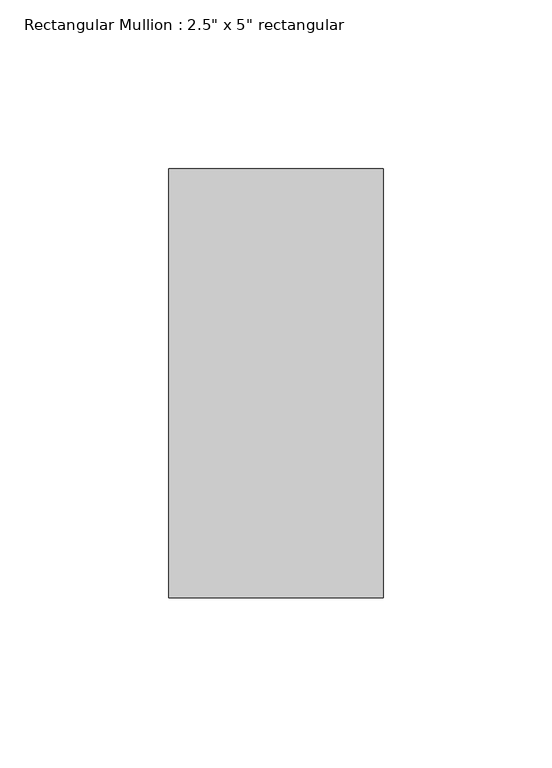
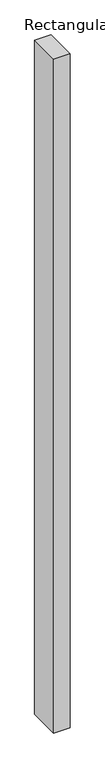
"""IFC4 building model written with IfcOpenShell, lengths in millimetres: member geometry."""

from ifc_helpers import new_model, si_unit, frame, origin, place, context, project, spatial, polyline, outline, extrude, source, transform, mapped, element, save


def member_a78380a5(model_context):
    return source(origin(), model_context, "Body", "SweptSolid", [
        extrude(outline(polyline([(0.0, 63.5), (0.0, -63.5), (-63.5, -63.5), (-63.5, 63.5), (0.0, 63.5)])), frame((0.0, 0.0, -2743.2), z_axis=(0.0, 0.0, 1.0), x_axis=(1.0, 0.0, 0.0)), (0.0, 0.0, 1.0), 2743.2),
    ])


if __name__ == "__main__":
    model = new_model("IFC4")
    model_context = context("Model", 3, world=origin())
    ifc_project = project(units=[si_unit("LENGTHUNIT", "METRE", prefix="MILLI")], contexts=[model_context])
    site = spatial("IfcSite", under=ifc_project)
    building = spatial("IfcBuilding", under=site)
    placement = place(None, origin())
    member_shape = member_a78380a5(model_context)
    element("IfcMember", 1, ObjectType="Rectangular Mullion : 2.5\" x 5\" rectangular", at=placement, inside=building, context=model_context, shape_type="MappedRepresentation", body=[
        mapped(member_shape, transform((0.0, 0.0, 0.0), x_axis=(1.0, 0.0, 0.0), y_axis=(0.0, 1.0, 0.0), z_axis=(0.0, 0.0, 1.0))),
    ])
    save(model, "model.ifc")

# Revit data of these elements
# Type "Rectangular Mullion : 2.5\" x 5\" rectangular"
#   built-in parameter 1007304 = 0.416667 (stored number, unit not read)
#   built-in parameter 1007301 = 0.104167 (stored number, unit not read)
#   built-in parameter 1007300 = 0.104167 (stored number, unit not read)
# Element 1 (IfcMember, "Rectangular Mullion : 2.5\" x 5\" rectangular")
#   Materials on its faces: "Aluminum"
# Materials
#   "Aluminum": class "Metal", colour RGB 247 247 247, transparency 0, Description = "Aluminum 6061", Cost = 0
